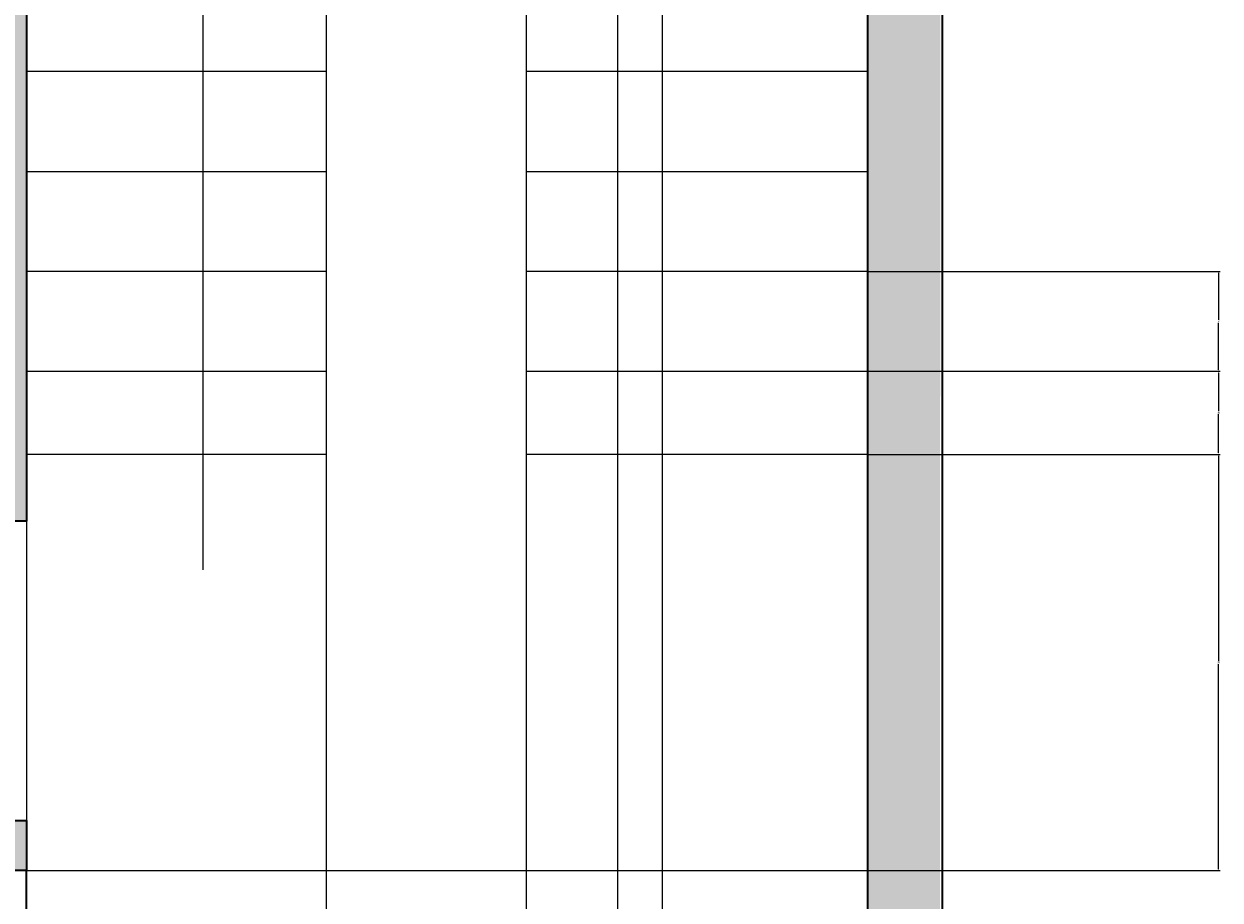
# Model space of a CAD drawing. Units: inches. Extents: x 2070 to 4408, y 1595 to 4269.
# Tile 7 of 20: x 2345 to 2489, y 1739 to 1844. Entities that reach past the tile are written whole.
import ezdxf

# ---------------------------------------------------------------- set-up
doc = ezdxf.new("R2010")
doc.units = ezdxf.units.IN
for name, color, linetype, lineweight in [('A-ANNO-DIMS', 2, 'Continuous', 18), ('A-ANNO-SYMB', 7, 'Continuous', 18), ('A-FLOR-STRS', 7, 'Continuous', 18), ('A-WALL', 7, 'Continuous', 35)]:
    doc.layers.add(name, color=color, linetype=linetype, lineweight=lineweight)
doc.layers.add('A-WALL-PATT', color=18, linetype='Continuous', lineweight=13, true_color=0x000000)
doc.styles.get("Standard").update_dxf_attribs({"font": 'arial.ttf'})
doc.dimstyles.get("Standard").update_dxf_attribs({"dimtxt": 0.18, "dimasz": 0.18, "dimexe": 0.18, "dimexo": 0.0625, "dimgap": 0.09, "dimtad": 0, "dimtih": 1, "dimtoh": 1, "dimdec": 4, "dimzin": 0, "dimdsep": 46, "dimtxsty": 'Standard', "dimcen": 0.09, "dimadec": 0, "dimazin": 0, "dimtfac": 1, "dimtdec": 4, "dimtofl": 0, "dimtmove": 0, "dimatfit": 3, "dimfxl": 1, "dimtolj": 1, "dimtzin": 0, "dimarcsym": 0})

# ---------------------------------------------------------------- blocks, each defined once
blk = doc.blocks.new('*D30')
at = {"layer": 'A-ANNO-DIMS', "color": 0, "lineweight": -2, "transparency": 16777216}
for p, q in [((2416.2, 2080.34), (2416.2, 1595.04)), ((2446.2, 2080.34), (2446.2, 1595.04)), ((2416.38, 1595.22), (2430.98, 1595.22)), ((2446.02, 1595.22), (2431.41, 1595.22))]:
    blk.add_line(p, q, dxfattribs=at)
at = {"layer": 'A-ANNO-DIMS', "color": 0, "transparency": 16777216}
for points in [[(2416.38, 1595.25), (2416.38, 1595.19), (2416.2, 1595.22)], [(2446.02, 1595.25), (2446.02, 1595.19), (2446.2, 1595.22)]]:
    blk.add_solid(points, dxfattribs=at)
at = {"layer": 'Defpoints', "color": 0, "transparency": 16777216}
for p in [(2416.2, 2080.4), (2446.2, 2080.4), (2446.2, 1595.22)]:
    blk.add_point(p, dxfattribs=at)
at = {"layer": 'A-ANNO-DIMS', "color": 0, "transparency": 16777216, "insert": (2431.2, 1595.22), "char_height": 0.18, "attachment_point": 5}
blk.add_mtext('\\A1;30', dxfattribs=at)
blk = doc.blocks.new('*D34')
at = {"layer": 'A-ANNO-DIMS', "color": 0, "lineweight": -2, "transparency": 16777216}
for p, q in [((2421.53, 2212.34), (2421.53, 1595.04)), ((2446.2, 2212.34), (2446.2, 1595.04)), ((2421.71, 1595.22), (2433.4, 1595.22)), ((2446.02, 1595.22), (2434.33, 1595.22))]:
    blk.add_line(p, q, dxfattribs=at)
at = {"layer": 'A-ANNO-DIMS', "color": 0, "transparency": 16777216}
for points in [[(2421.71, 1595.25), (2421.71, 1595.19), (2421.53, 1595.22)], [(2446.02, 1595.25), (2446.02, 1595.19), (2446.2, 1595.22)]]:
    blk.add_solid(points, dxfattribs=at)
at = {"layer": 'Defpoints', "color": 0, "transparency": 16777216}
for p in [(2421.53, 2212.4), (2446.2, 2212.4), (2446.2, 1595.22)]:
    blk.add_point(p, dxfattribs=at)
at = {"layer": 'A-ANNO-DIMS', "color": 0, "transparency": 16777216, "insert": (2433.86, 1595.22), "char_height": 0.18, "attachment_point": 5}
blk.add_mtext('\\A1;24.663', dxfattribs=at)
blk = doc.blocks.new('*D36')
at = {"layer": 'A-ANNO-DIMS', "color": 0, "lineweight": -2, "transparency": 16777216}
for p, q in [((2345.2, 1792.34), (2345.2, 1595.04)), ((2381.2, 1792.34), (2381.2, 1595.04)), ((2345.38, 1595.22), (2362.98, 1595.22)), ((2381.02, 1595.22), (2363.41, 1595.22))]:
    blk.add_line(p, q, dxfattribs=at)
at = {"layer": 'A-ANNO-DIMS', "color": 0, "transparency": 16777216}
for points in [[(2345.38, 1595.25), (2345.38, 1595.19), (2345.2, 1595.22)], [(2381.02, 1595.25), (2381.02, 1595.19), (2381.2, 1595.22)]]:
    blk.add_solid(points, dxfattribs=at)
at = {"layer": 'Defpoints', "color": 0, "transparency": 16777216}
for p in [(2345.2, 1792.4), (2381.2, 1792.4), (2381.2, 1595.22)]:
    blk.add_point(p, dxfattribs=at)
at = {"layer": 'A-ANNO-DIMS', "color": 0, "transparency": 16777216, "insert": (2363.2, 1595.22), "char_height": 0.18, "attachment_point": 5}
blk.add_mtext('\\A1;36', dxfattribs=at)
blk = doc.blocks.new('*D37')
at = {"layer": 'A-ANNO-DIMS', "color": 0, "lineweight": -2, "transparency": 16777216}
for p, q in [((2381.2, 1792.34), (2381.2, 1595.04)), ((2405.2, 1792.34), (2405.2, 1595.04)), ((2381.38, 1595.22), (2392.98, 1595.22)), ((2405.02, 1595.22), (2393.42, 1595.22))]:
    blk.add_line(p, q, dxfattribs=at)
at = {"layer": 'A-ANNO-DIMS', "color": 0, "transparency": 16777216}
for points in [[(2381.38, 1595.25), (2381.38, 1595.19), (2381.2, 1595.22)], [(2405.02, 1595.25), (2405.02, 1595.19), (2405.2, 1595.22)]]:
    blk.add_solid(points, dxfattribs=at)
at = {"layer": 'Defpoints', "color": 0, "transparency": 16777216}
for p in [(2381.2, 1792.4), (2405.2, 1792.4), (2405.2, 1595.22)]:
    blk.add_point(p, dxfattribs=at)
at = {"layer": 'A-ANNO-DIMS', "color": 0, "transparency": 16777216, "insert": (2393.2, 1595.22), "char_height": 0.18, "attachment_point": 5}
blk.add_mtext('\\A1;24', dxfattribs=at)
blk = doc.blocks.new('*D38')
at = {"layer": 'A-ANNO-DIMS', "color": 0, "lineweight": -2, "transparency": 16777216}
for p, q in [((2405.2, 1792.34), (2405.2, 1595.04)), ((2446.2, 1792.34), (2446.2, 1595.04)), ((2405.38, 1595.22), (2425.49, 1595.22)), ((2446.02, 1595.22), (2425.9, 1595.22))]:
    blk.add_line(p, q, dxfattribs=at)
at = {"layer": 'A-ANNO-DIMS', "color": 0, "transparency": 16777216}
for points in [[(2405.38, 1595.25), (2405.38, 1595.19), (2405.2, 1595.22)], [(2446.02, 1595.25), (2446.02, 1595.19), (2446.2, 1595.22)]]:
    blk.add_solid(points, dxfattribs=at)
at = {"layer": 'Defpoints', "color": 0, "transparency": 16777216}
for p in [(2405.2, 1792.4), (2446.2, 1792.4), (2446.2, 1595.22)]:
    blk.add_point(p, dxfattribs=at)
at = {"layer": 'A-ANNO-DIMS', "color": 0, "transparency": 16777216, "insert": (2425.7, 1595.22), "char_height": 0.18, "attachment_point": 5}
blk.add_mtext('\\A1;41', dxfattribs=at)
blk = doc.blocks.new('*D39')
at = {"layer": 'A-ANNO-DIMS', "color": 0, "lineweight": -2, "transparency": 16777216}
for p, q in [((2446.26, 1814.4), (2488.56, 1814.4)), ((2488.38, 1814.22), (2488.38, 1808.58)), ((2488.38, 1802.58), (2488.38, 1808.22)), ((2446.26, 1802.4), (2488.56, 1802.4))]:
    blk.add_line(p, q, dxfattribs=at)
at = {"layer": 'A-ANNO-DIMS', "color": 0, "transparency": 16777216}
for points in [[(2488.35, 1814.22), (2488.41, 1814.22), (2488.38, 1814.4)], [(2488.35, 1802.58), (2488.41, 1802.58), (2488.38, 1802.4)]]:
    blk.add_solid(points, dxfattribs=at)
at = {"layer": 'Defpoints', "color": 0, "transparency": 16777216}
for p in [(2446.2, 1814.4), (2446.2, 1802.4), (2488.38, 1802.4)]:
    blk.add_point(p, dxfattribs=at)
at = {"layer": 'A-ANNO-DIMS', "color": 0, "transparency": 16777216, "insert": (2488.38, 1808.4), "char_height": 0.18, "attachment_point": 5}
blk.add_mtext('\\A1;12', dxfattribs=at)
blk = doc.blocks.new('*D40')
at = {"layer": 'A-ANNO-DIMS', "color": 0, "lineweight": -2, "transparency": 16777216}
for p, q in [((2446.26, 1802.4), (2488.56, 1802.4)), ((2488.38, 1802.22), (2488.38, 1797.58)), ((2488.38, 1792.58), (2488.38, 1797.22)), ((2446.26, 1792.4), (2488.56, 1792.4))]:
    blk.add_line(p, q, dxfattribs=at)
at = {"layer": 'A-ANNO-DIMS', "color": 0, "transparency": 16777216}
for points in [[(2488.35, 1802.22), (2488.41, 1802.22), (2488.38, 1802.4)], [(2488.35, 1792.58), (2488.41, 1792.58), (2488.38, 1792.4)]]:
    blk.add_solid(points, dxfattribs=at)
at = {"layer": 'Defpoints', "color": 0, "transparency": 16777216}
for p in [(2446.2, 1802.4), (2446.2, 1792.4), (2488.38, 1792.4)]:
    blk.add_point(p, dxfattribs=at)
at = {"layer": 'A-ANNO-DIMS', "color": 0, "transparency": 16777216, "insert": (2488.38, 1797.4), "char_height": 0.18, "attachment_point": 5}
blk.add_mtext('\\A1;10', dxfattribs=at)
blk = doc.blocks.new('*D42')
at = {"layer": 'A-ANNO-DIMS', "color": 0, "lineweight": -2, "transparency": 16777216}
for p, q in [((2446.26, 1792.4), (2488.56, 1792.4)), ((2488.38, 1792.22), (2488.38, 1767.58)), ((2488.38, 1742.58), (2488.38, 1767.22)), ((2446.26, 1742.4), (2488.56, 1742.4))]:
    blk.add_line(p, q, dxfattribs=at)
at = {"layer": 'A-ANNO-DIMS', "color": 0, "transparency": 16777216}
for points in [[(2488.35, 1792.22), (2488.41, 1792.22), (2488.38, 1792.4)], [(2488.35, 1742.58), (2488.41, 1742.58), (2488.38, 1742.4)]]:
    blk.add_solid(points, dxfattribs=at)
at = {"layer": 'Defpoints', "color": 0, "transparency": 16777216}
for p in [(2446.2, 1792.4), (2488.38, 1792.4), (2446.2, 1742.4)]:
    blk.add_point(p, dxfattribs=at)
at = {"layer": 'A-ANNO-DIMS', "color": 0, "transparency": 16777216, "insert": (2488.38, 1767.4), "char_height": 0.18, "attachment_point": 5}
blk.add_mtext('\\A1;50', dxfattribs=at)

msp = doc.modelspace()

# ---------------------------------------------------------------- hatches: boundary and pattern name
at = {"layer": 'A-WALL-PATT'}
h = msp.add_hatch(color=256, dxfattribs=at)
h.dxf.hatch_style = 1
h.paths.add_polyline_path([(2346.196, 2218.3995), (2346.196, 2282.3995), (2340.196, 2282.3995), (2340.196, 2212.3995), (2345.5866, 2212.3995), (2346.196, 2212.3995)], flags=0)
h.paths.add_polyline_path([(2245.196, 2282.3995), (2239.196, 2282.3995), (2239.196, 2186.3995), (2244.5866, 2186.3995), (2245.196, 2186.3995)], flags=0)
h.paths.add_polyline_path([(2340.196, 2230.6455), (2245.196, 2230.6455), (2245.196, 2224.6455), (2340.196, 2224.6455)], flags=0)
h.paths.add_polyline_path([(2245.196, 2150.3995), (2239.196, 2150.3995), (2164.4362, 2150.3995), (2164.4362, 2144.3995), (2239.196, 2144.3995), (2239.196, 2086.3995), (2239.196, 2067.2711), (2244.5866, 2067.2711), (2245.196, 2067.2711), (2245.196, 2144.3995)], flags=0)
h.paths.add_polyline_path([(2346.196, 2176.3995), (2340.196, 2176.3995), (2340.196, 2086.3995), (2346.196, 2086.3995), (2346.196, 2125.318)], flags=0)
h.paths.add_polyline_path([(2446.196, 2086.3995), (2346.196, 2086.3995), (2340.196, 2086.3995), (2340.196, 2080.3995), (2446.196, 2080.3995)], flags=0)
h.paths.add_polyline_path([(2455.196, 2291.3995), (2103.196, 2291.3995), (2103.196, 1699.3995), (2336.196, 1699.3995), (2336.196, 1628.3995), (2345.196, 1628.3995), (2446.196, 1628.3995), (2454.8846, 1628.3995), (2454.8846, 1699.3995)])
h.paths.add_polyline_path([(2446.196, 2282.3995), (2446.196, 2218.3995), (2446.196, 2212.3995), (2446.196, 2086.3995), (2446.196, 2080.3995), (2446.196, 1708.3995), (2446.196, 1637.3995), (2345.196, 1637.3995), (2345.196, 1699.3995), (2345.196, 1708.3995), (2336.196, 1708.3995), (2112.196, 1708.3995), (2112.196, 2282.3995), (2239.196, 2282.3995), (2245.196, 2282.3995), (2356.196, 2282.3995)], flags=16)
h.paths.add_polyline_path([(2245.196, 2150.3995), (2245.196, 2144.3995), (2245.196, 2067.2711), (2244.5866, 2067.2711), (2239.196, 2067.2711), (2239.196, 2065.6988), (2203.2929, 2065.6988, 0.40145271), (2239.196, 2031.3337), (2244.5866, 2031.3337), (2245.196, 2031.2711), (2245.196, 1924.1525), (2239.196, 1924.1525), (2239.196, 1922.5803), (2203.2929, 1922.5803, 0.40145271), (2239.196, 1888.2151), (2244.5866, 1888.2151), (2245.196, 1888.1525), (2245.196, 1748.3995), (2339.196, 1748.4621, -0.40145271), (2303.2929, 1782.8272), (2303.2585, 1782.8272), (2303.2585, 1784.3995), (2339.196, 1784.3995), (2339.196, 1877.2067), (2291.196, 1877.2067), (2291.196, 1883.2067), (2291.196, 1946.3995), (2291.196, 1952.3995), (2291.196, 2086.3995), (2297.196, 2086.3995), (2302.196, 2086.3995), (2302.196, 2081.0259), (2303.7633, 2081.0259), (2303.7633, 2080.3995), (2338.0148, 2080.3995, 0.00437129), (2338.0203, 2081.0259), (2338.0203, 2086.3995), (2340.196, 2086.3995), (2340.196, 2176.4621), (2345.5866, 2176.4621, 0.40145271), (2381.4896, 2210.8272), (2345.5866, 2210.8272), (2345.5866, 2212.3995), (2340.196, 2212.3995), (2340.196, 2224.6455), (2245.196, 2224.6455), (2245.196, 2186.3995), (2244.5866, 2186.3995), (2239.196, 2186.3995), (2239.196, 2184.8272), (2203.2929, 2184.8272, 0.40145271), (2239.196, 2150.4621), (2244.5866, 2150.4621)], flags=0)
h.paths.add_polyline_path([(2346.196, 2282.3995), (2346.196, 2218.3995), (2377.1813, 2218.3995), (2377.1813, 2212.3995), (2346.196, 2212.3995), (2345.5866, 2212.3995), (2340.196, 2212.3995), (2340.196, 2224.6455), (2245.196, 2224.6455), (2245.196, 2230.6455), (2245.196, 2282.3995), (2292.696, 2256.5225), (2340.196, 2282.3995)], flags=0)
h.paths.add_polyline_path([(2346.196, 2086.3995), (2340.196, 2086.3995), (2340.196, 2080.3995), (2446.196, 2080.3995), (2431.196, 2016.3995), (2446.196, 1952.3995), (2412.196, 1952.3995), (2412.196, 2080.3995), (2340.196, 2080.3995), (2340.196, 2086.3995), (2340.196, 2176.3995), (2346.196, 2176.3995), (2346.196, 2125.318)], flags=0)
h.paths.add_polyline_path([(2186.508, 2270.0471, -0.03755288), (2186.9712, 2269.8581), (2186.9164, 2270.112, -0.02759121)], flags=0)
h.paths.add_polyline_path([(2183.955, 2273.7766, 1), (2188.2945, 2273.7766, 1)], flags=0)
h.paths.add_polyline_path([(2142.5261, 2274.6158, -0.03707541), (2142.5672, 2275.1696), (2142.5672, 2276.826), (2119.8759, 2276.826), (2119.8759, 2263.0962), (2140.4332, 2263.0962), (2142.5672, 2263.0962), (2142.5672, 2274.0621, -0.03707541)], flags=0)
h.paths.add_polyline_path([(2209.8974, 2263.0962), (2209.8974, 2262.2079), (2190.8042, 2262.2079), (2190.8042, 2263.0962)], flags=0)
h.paths.add_polyline_path([(2210.6382, 2276.1833), (2210.6382, 2263.9844), (2190.2185, 2263.9844), (2190.2185, 2276.1833)], flags=0)
h.paths.add_polyline_path([(2188.4362, 2273.7766, -1), (2183.8133, 2273.7766, -1)], flags=0)
h.paths.add_polyline_path([(2245.196, 2150.3995), (2245.196, 2144.3995), (2245.196, 2067.2711), (2239.196, 2067.2711), (2239.196, 2080.3995), (2172.196, 2080.3995), (2172.196, 2000.3995), (2239.196, 2000.3995), (2239.196, 1940.3995), (2159.0187, 1940.3995), (2123.0187, 1940.3995), (2112.196, 1940.3995), (2112.196, 1946.3995), (2123.0187, 1946.3995), (2123.0187, 1982.2238), (2124.586, 1982.2238), (2124.586, 1982.1895, -0.40145271), (2158.8429, 1946.3995), (2159.0187, 1946.3995), (2239.196, 1946.3995), (2239.196, 1994.3995), (2112.196, 1994.3995), (2112.196, 2000.3995), (2139.196, 2040.3995), (2112.196, 2080.3995), (2112.196, 2086.3995), (2239.196, 2086.3995), (2239.196, 2144.3995), (2209.5809, 2144.3995), (2209.5809, 2136.3995), (2203.0809, 2136.3995), (2205.0809, 2130.3996, -0.70257121), (2199.081, 2116.3995, -0.70256205), (2193.0809, 2130.3994), (2195.0809, 2136.3995), (2192.0809, 2136.3995), (2192.0809, 2134.8995), (2189.0809, 2134.8995), (2189.0809, 2135.8995), (2191.0809, 2135.8995), (2191.0809, 2136.3995), (2188.5809, 2136.3995), (2188.5809, 2144.3995), (2164.2481, 2144.3995, -0.39385849), (2130.0035, 2109.5491), (2130.0035, 2109.5147), (2128.4362, 2109.5147), (2128.4362, 2144.3995), (2112.196, 2144.3995), (2112.196, 2150.3995), (2128.4362, 2150.3995), (2128.4362, 2150.7127), (2164.4362, 2150.7127), (2164.4362, 2150.3995), (2239.196, 2150.3995)], flags=0)
h.paths.add_polyline_path([(2188.2075, 2266.8735), (2188.2075, 2211.8632, -0.41421356), (2185.4833, 2209.1391), (2146.7995, 2209.1391, -0.41421356), (2144.0754, 2211.8632), (2144.0754, 2266.8735, -0.41421356), (2146.7995, 2269.5976), (2185.4833, 2269.5976, -0.41421356)], flags=0)
h.paths.add_polyline_path([(2185.0844, 2273.7766, -1), (2187.1651, 2273.7766, -1)], flags=0)
h.paths.add_polyline_path([(2182.0486, 2259.2932), (2168.0953, 2259.2932), (2168.0953, 2260.8424), (2163.7261, 2260.8424), (2163.7261, 2259.2932), (2149.7727, 2259.2932), (2149.7727, 2266.3352), (2163.7261, 2266.3352), (2163.7261, 2261.9839), (2168.0953, 2261.9839), (2168.0953, 2266.3352), (2182.0486, 2266.3352)], flags=0)
h.paths.add_polyline_path([(2148.2585, 2250.2051), (2153.0615, 2241.8861, 0.39807048)], flags=0)
h.paths.add_polyline_path([(2162.7572, 2247.2885), (2153.1461, 2241.7396), (2148.1083, 2250.4653), (2157.7194, 2256.0142)], flags=0)
h.paths.add_polyline_path([(2162.6726, 2247.4351, -0.39286196), (2157.8415, 2255.6313), (2157.6431, 2255.6313), (2157.8696, 2255.7541)], flags=0)
h.paths.add_polyline_path([(2164.2604, 2145.339), (2164.4362, 2144.3995), (2164.4362, 2150.3995), (2164.2604, 2150.7127)], flags=0)
h.paths.add_polyline_path([(2208.5809, 2142.6495), (2208.5809, 2138.3995, -0.41421356), (2207.8309, 2137.3995), (2190.5809, 2137.3995, -0.41421356), (2189.5809, 2138.1495), (2189.5809, 2142.3995, -0.41421356), (2190.3309, 2143.3995), (2207.5809, 2143.3995, -0.41421356)], flags=0)
h.paths.add_polyline_path([(2147.957, 2229.9119), (2154.7494, 2223.1195, 0.39807048)], flags=0)
h.paths.add_polyline_path([(2162.7165, 2230.8473), (2154.8691, 2222.9998), (2147.7446, 2230.1244), (2155.592, 2237.9718)], flags=0)
h.paths.add_polyline_path([(2162.5969, 2230.9669, -0.39807048), (2155.8044, 2237.7594)], flags=0)
h.paths.add_polyline_path([(2391.8776, 2049.9192), (2408.5766, 2049.9192), (2408.5766, 2033.2202), (2408.5766, 1983.123), (2408.5766, 1966.4239), (2391.8776, 1966.4239), (2391.8776, 1983.123), (2341.7804, 1983.123), (2341.7804, 2033.2202), (2391.8776, 2033.2202)], flags=0)
h.paths.add_polyline_path([(2144.1055, 2274.6158, 1), (2148.445, 2274.6158, 1)], flags=0)
h.paths.add_polyline_path([(2148.5867, 2274.6158, -1), (2143.9638, 2274.6158, -1)], flags=0)
h.paths.add_polyline_path([(2145.2349, 2274.6158, -1), (2147.3156, 2274.6158, -1)], flags=0)
edge = h.paths.add_edge_path(flags=0)
edge.add_ellipse((2400.5951, 2040.9436), major_axis=(-4.5109, 0), ratio=0.97544784, start_angle=180, end_angle=270, ccw=False)
edge.add_ellipse((2400.5951, 2040.9436), major_axis=(-4.5109, 0), ratio=0.97544784, start_angle=90, end_angle=180, ccw=False)
edge.add_ellipse((2400.5951, 2040.9436), major_axis=(-4.5109, 0), ratio=0.97544784, start_angle=0, end_angle=90, ccw=False)
edge.add_ellipse((2400.5951, 2040.9436), major_axis=(-4.5109, 0), ratio=0.97544784, start_angle=270, end_angle=360, ccw=False)
h.paths.add_polyline_path([(2199.0809, 2117.3995, -0.73452973), (2195.0809, 2130.3995), (2203.081, 2130.3995, -0.73453329)], flags=0)
h.paths.add_polyline_path([(2141.9147, 2276.0353), (2141.9147, 2263.9844), (2120.4685, 2263.9844), (2120.4685, 2276.0353)], flags=0)
h.paths.add_polyline_path([(2138.4481, 2273.4072), (2138.4481, 2266.7226), (2133.2801, 2266.7226), (2133.2801, 2273.4072)], flags=0)
h.paths.add_polyline_path([(2137.9691, 2272.9175), (2137.9691, 2272.204), (2135.4229, 2272.204), (2135.4229, 2271.6329), (2135.3221, 2270.1051), (2135.3221, 2269.0265), (2135.4229, 2268.6811), (2135.4229, 2267.2011), (2133.7212, 2267.2011), (2133.7212, 2268.6811), (2133.7983, 2269.9587), (2133.7983, 2271.2758), (2133.7212, 2271.6329), (2133.7212, 2273.0065), (2135.717, 2273.0065), (2135.717, 2272.9175)], flags=0)
h.paths.add_polyline_path([(2137.9215, 2271.8264), (2137.9215, 2271.3786), (2137.5182, 2271.3786), (2136.9355, 2271.3786), (2136.3529, 2271.3786), (2135.7703, 2271.3786), (2135.7703, 2271.8264), (2136.1736, 2271.8264), (2136.7562, 2271.8264), (2137.3389, 2271.8264)], flags=0)
h.paths.add_polyline_path([(2137.9215, 2271.692), (2137.5182, 2271.692), (2136.9355, 2271.513), (2137.3389, 2271.513)], flags=0)
h.paths.add_polyline_path([(2136.3529, 2271.692), (2135.7703, 2271.513), (2136.1736, 2271.513), (2136.7562, 2271.692)], flags=0)
h.paths.add_polyline_path([(2137.9215, 2271.513), (2137.5182, 2271.513), (2136.7562, 2271.747), (2136.7562, 2271.692), (2137.3389, 2271.692)], flags=0)
h.paths.add_polyline_path([(2137.8207, 2270.4664), (2137.8207, 2270.0971), (2137.8207, 2269.627), (2137.8207, 2269.1569), (2137.8207, 2268.6868), (2137.3837, 2268.6868), (2136.6442, 2268.6868), (2135.9271, 2268.6868), (2135.9271, 2269.0562), (2135.9271, 2269.5263), (2135.9271, 2269.9963), (2135.9271, 2270.4664), (2136.3641, 2270.4664), (2137.0812, 2270.4664)], flags=0)
h.paths.add_polyline_path([(2137.3837, 2269.627), (2137.8207, 2269.627), (2137.8207, 2269.5263), (2137.3837, 2269.5263), (2137.3837, 2269.1569), (2137.8207, 2269.1569), (2137.3837, 2269.0562), (2137.3837, 2268.6868), (2137.0812, 2268.6868), (2137.0812, 2269.0562), (2136.6442, 2269.0562), (2136.6442, 2268.6868), (2136.3641, 2268.6868), (2136.3641, 2269.0562), (2135.9271, 2269.0562), (2135.9271, 2269.1569), (2136.3641, 2269.1569), (2136.3641, 2269.5263), (2135.9271, 2269.5263), (2135.9271, 2269.627), (2136.3641, 2269.627), (2136.3641, 2269.9963), (2135.9271, 2269.9963), (2136.3641, 2270.0971), (2136.3641, 2270.4664), (2136.6442, 2270.4664), (2136.6442, 2270.0971), (2137.0812, 2270.0971), (2137.0812, 2270.4664), (2137.3837, 2270.4664), (2137.3837, 2270.0971), (2137.8207, 2270.0971), (2137.3837, 2269.9963)], flags=0)
h.paths.add_polyline_path([(2137.5182, 2271.8264), (2137.5182, 2271.692), (2137.3389, 2271.3786), (2137.3389, 2271.513)], flags=0)
h.paths.add_polyline_path([(2137.8179, 2267.8138), (2137.8179, 2267.6879), (2137.1876, 2267.6879), (2136.4733, 2267.6879), (2135.759, 2267.6879), (2135.759, 2267.8138), (2136.3893, 2267.8138), (2137.1036, 2267.8138)], flags=0)
h.paths.add_polyline_path([(2137.0812, 2269.9963), (2137.0812, 2269.627), (2137.0812, 2269.1569), (2136.6442, 2269.1569), (2136.6442, 2269.5263), (2136.6442, 2269.9963)], flags=0)
h.paths.add_polyline_path([(2136.3529, 2271.8264), (2136.3529, 2271.692), (2136.1736, 2271.3786), (2136.1736, 2271.513)], flags=0)
h.paths.add_polyline_path([(2136.4733, 2267.8138), (2136.4733, 2267.6879), (2136.3893, 2267.6879), (2136.3893, 2267.8138)], flags=0)
h.paths.add_polyline_path([(2407.9087, 2032.5522), (2407.9087, 1983.7909), (2359.81, 1983.7909, -0.00912788), (2359.0575, 1983.7909), (2342.4483, 1983.7909), (2342.4483, 2032.5522)], flags=0)
h.paths.add_polyline_path([(2389.1838, 2023.1358), (2353.7856, 2023.1358), (2353.7856, 1985.4867, -0.09210376), (2350.2788, 1988.655), (2350.2788, 2026.6426), (2389.1838, 2026.6426)], flags=0)
h.paths.add_polyline_path([(2352.6166, 2024.3048), (2351.4477, 2024.3048), (2351.4477, 2025.4737), (2352.6166, 2025.4737)], flags=0)
h.paths.add_polyline_path([(2399.6319, 2026.7589), (2404.3661, 2026.7589, -0.41421356), (2407.0379, 2024.087), (2407.0379, 2013.4908, -0.41421356), (2404.3661, 2010.819), (2399.6319, 2010.819, -0.41421356), (2396.96, 2013.4908), (2396.96, 2024.087, -0.41421356)], flags=0)
h.paths.add_polyline_path([(2399.6319, 2026.0909), (2404.3661, 2026.0909, -0.41421356), (2406.37, 2024.087), (2406.37, 2013.4908, -0.41421356), (2404.3661, 2011.487), (2399.6319, 2011.487, -0.41421356), (2397.628, 2013.4908), (2397.628, 2024.087, -0.41421356)], flags=0)
h.paths.add_polyline_path([(2399.6319, 2002.3217), (2404.3661, 2002.3217, -0.41421356), (2407.0379, 1999.6498), (2407.0379, 1989.0536, -0.41421356), (2404.3661, 1986.3818), (2399.6319, 1986.3818, -0.41421356), (2396.96, 1989.0536), (2396.96, 1999.6498, -0.41421356)], flags=0)
h.paths.add_polyline_path([(2399.6319, 2001.6537), (2404.3661, 2001.6537, -0.41421356), (2406.37, 1999.6498), (2406.37, 1989.0536, -0.41421356), (2404.3661, 1987.0497), (2399.6319, 1987.0497, -0.41421356), (2397.628, 1989.0536), (2397.628, 1999.6498, -0.41421356)], flags=0)
edge = h.paths.add_edge_path(flags=0)
edge.add_ellipse((2400.5951, 1975.3996), major_axis=(-4.5109, 0), ratio=0.97544784, start_angle=-180, end_angle=-90, ccw=False)
edge.add_ellipse((2400.5951, 1975.3996), major_axis=(-4.5109, 0), ratio=0.97544784, start_angle=90, end_angle=180, ccw=False)
edge.add_ellipse((2400.5951, 1975.3996), major_axis=(-4.5109, 0), ratio=0.97544784, start_angle=0, end_angle=90, ccw=False)
edge.add_ellipse((2400.5951, 1975.3996), major_axis=(-4.5109, 0), ratio=0.97544784, start_angle=-90, end_angle=0, ccw=False)
h.paths.add_polyline_path([(2345.196, 1910.3995), (2366.4386, 1910.3995), (2366.4386, 1925.4555), (2392.3856, 1925.4555), (2392.3856, 1933.5025), (2400.1399, 1925.4555), (2392.3856, 1919.8795), (2392.3856, 1925.4555), (2366.4386, 1925.4555), (2366.4386, 1910.3995), (2381.196, 1910.3995), (2405.196, 1910.3995), (2405.196, 1898.3995), (2446.196, 1898.3995), (2446.196, 1886.3995), (2405.196, 1886.3995), (2405.196, 1874.3995), (2446.196, 1874.3995), (2446.196, 1862.3995), (2405.196, 1862.3995), (2405.196, 1850.3995), (2446.196, 1850.3995), (2446.196, 1838.3995), (2405.196, 1838.3995), (2405.196, 1826.3995), (2446.196, 1826.3995), (2446.196, 1814.3995), (2405.196, 1814.3995), (2405.196, 1802.3995), (2446.196, 1802.3995), (2446.196, 1798.3995), (2446.196, 1792.3995), (2405.196, 1792.3995), (2405.196, 1910.3995), (2381.196, 1910.3995), (2381.196, 1792.3995), (2345.196, 1792.3995)], flags=0)
h.paths.add_polyline_path([(2333.0944, 1863.3993, -0.41421356), (2334.7225, 1861.7712), (2334.7225, 1859.329), (2335.2653, 1859.329, -0.41421356), (2337.4361, 1857.1582), (2337.4361, 1843.862, -0.41421356), (2335.2653, 1841.6911, -0.41421356), (2337.4361, 1839.5203), (2337.4361, 1827.5808, -0.41421356), (2335.2653, 1825.41, -0.41421356), (2337.4361, 1823.2392), (2337.4361, 1808.5862, -0.41421356), (2335.2653, 1806.4153), (2334.7225, 1806.4153), (2334.7225, 1803.9732, -0.41421356), (2333.0944, 1802.3451), (2317.356, 1802.3451), (2317.0846, 1802.3451, -0.41421356), (2315.7279, 1803.7018), (2315.7279, 1803.8646), (2313.8284, 1803.8646, -0.41421356), (2311.6576, 1806.0354), (2311.6576, 1823.2015, -0.39597602), (2313.6834, 1825.3765, -0.43384798), (2311.6576, 1827.2718), (2311.6576, 1839.761, -0.41421356), (2313.5571, 1841.6604), (2313.8284, 1841.6604), (2333.8159, 1841.6604, -0.04213623), (2334.1798, 1841.6911, -0.41421356), (2332.009, 1843.862), (2332.009, 1857.1582, -0.41421356), (2334.1798, 1859.329), (2317.356, 1859.329), (2317.0846, 1859.329, -0.41421356), (2315.7279, 1860.6858), (2315.7279, 1862.0426, -0.41421356), (2317.0846, 1863.3993), (2317.356, 1863.3993)], flags=0)
h.paths.add_polyline_path([(2208.8475, 1848.9818), (2208.8475, 1840.9741, -0.41421356), (2207.0458, 1839.1724), (2206.5453, 1839.1721), (2206.5453, 1838.7218, -0.40985861), (2204.7704, 1836.9203), (2183.7501, 1836.9203, -0.41858196), (2181.9216, 1838.7218), (2181.9216, 1839.1721), (2181.421, 1839.1724, -0.41421356), (2179.6193, 1840.9741), (2179.6193, 1848.6817, -0.44064415), (2185.1126, 1854.9874), (2203.3852, 1854.9874, -0.45707961)], flags=0)
h.paths.add_polyline_path([(2204.243, 1848.4815), (2204.243, 1848.4815, 0.41725335), (2202.2204, 1850.4833), (2186.2049, 1850.4833, 0.4111805), (2184.2237, 1848.4815), (2184.2237, 1848.4815, -0.4111807), (2186.2049, 1850.4833), (2202.2204, 1850.4833, -0.41725315)], flags=0)
h.paths.add_polyline_path([(2234.7177, 1830.228), (2234.7176, 1781.6047, -0.41421356), (2233.4381, 1780.3252), (2218.6064, 1780.3252, -0.41421356), (2217.8387, 1781.0929), (2217.8387, 1783.3961, -0.41421356), (2218.6064, 1784.1639), (2218.6065, 1796.9595, -0.41421356), (2219.886, 1798.239, -0.41421356), (2218.6065, 1799.5186), (2218.6065, 1812.3142, -0.41421356), (2219.8861, 1813.5938, -0.41421356), (2218.6065, 1814.8733), (2218.6065, 1827.6689, -0.41421356), (2217.8388, 1828.4367), (2217.8388, 1830.7399, -0.41421356), (2218.6065, 1831.5076), (2233.4382, 1831.5076, -0.41421356)], flags=0)
h.paths.add_polyline_path([(2230.6344, 1827.6689, -0.41421356), (2231.4021, 1826.9012), (2231.4021, 1784.9316, -0.41421356), (2230.6343, 1784.1639), (2221.1853, 1784.1639), (2221.1853, 1827.6689)], flags=0)
h.paths.add_polyline_path([(2222.7208, 1798.239), (2221.6971, 1798.239), (2221.6971, 1813.5938), (2222.7208, 1813.5938)], flags=0)
h.paths.add_polyline_path([(2206.5453, 1773.935), (2206.5453, 1773.4848), (2206.9457, 1773.4848), (2207.0458, 1773.4845, -0.41421356), (2208.8475, 1771.6827), (2208.8475, 1763.675, -0.44222432), (2203.6505, 1757.6695), (2185.3851, 1757.6695, -0.45508402), (2179.6193, 1763.9752), (2179.6193, 1771.6827, -0.41421356), (2181.421, 1773.4845), (2181.421, 1773.4848), (2181.9216, 1773.4848), (2181.9216, 1773.935, -0.40985861), (2183.6965, 1775.7366), (2204.7167, 1775.7366, -0.41858196)], flags=0)
h.paths.add_polyline_path([(2202.2619, 1762.1736), (2186.2464, 1762.1736, -0.41725315), (2184.2237, 1764.1754), (2184.2237, 1764.1754, 0.41725335), (2186.2464, 1762.1736), (2202.2619, 1762.1736, 0.4111805), (2204.243, 1764.1754), (2204.243, 1764.1754, -0.4111807)], flags=0)
h.paths.add_polyline_path([(2313.0034, 1713.1906), (2312.997, 1713.1697), (2313.0123, 1713.1612)], flags=0)
h.paths.add_polyline_path([(2305.7314, 1721.0488), (2305.6257, 1721.1994), (2305.4853, 1721.084)], flags=0)
h.paths.add_polyline_path([(2307.5562, 1726.1427), (2307.6186, 1726.1026), (2307.5737, 1726.0477), (2308.5692, 1720.6434), (2310.5345, 1721.2985), (2310.5721, 1721.411), (2310.6958, 1721.3523), (2313.8453, 1722.4021), (2314.9351, 1723.8033), (2314.9294, 1723.9165), (2315.0028, 1723.8903), (2313.874, 1722.4389), (2313.8697, 1722.4102), (2308.5692, 1720.6434), (2308.9864, 1720.122), (2309.0665, 1720.0971), (2309.053, 1720.0387), (2310.9235, 1717.7005), (2311.4182, 1717.6259), (2311.2918, 1717.2402), (2312.0655, 1716.2731), (2312.1081, 1716.2606), (2312.0969, 1716.2339), (2308.5692, 1720.6434), (2305.2249, 1717.745), (2305.232, 1717.704), (2305.1665, 1717.6944), (2308.5692, 1720.6434)], flags=0)
h.paths.add_polyline_path([(2288.2072, 1714.3431), (2288.2008, 1714.3222), (2288.216, 1714.3137)], flags=0)
h.paths.add_polyline_path([(2280.9352, 1722.2013), (2280.8295, 1722.3519), (2280.689, 1722.2365)], flags=0)
h.paths.add_polyline_path([(2282.76, 1727.2952), (2282.8224, 1727.2551), (2282.7775, 1727.2002), (2283.773, 1721.7959), (2285.7383, 1722.451), (2285.7759, 1722.5635), (2285.8995, 1722.5048), (2289.0491, 1723.5546), (2290.1389, 1724.9558), (2290.1332, 1725.069), (2290.2065, 1725.0428), (2289.0777, 1723.5915), (2289.0735, 1723.5628), (2283.773, 1721.7959), (2284.1901, 1721.2745), (2284.2703, 1721.2496), (2284.2567, 1721.1913), (2286.1273, 1718.8531), (2286.622, 1718.7785), (2286.4956, 1718.3927), (2287.2692, 1717.4256), (2287.3119, 1717.4131), (2287.3006, 1717.3864), (2283.773, 1721.7959), (2280.4286, 1718.8975), (2280.4357, 1718.8565), (2280.3703, 1718.8469), (2283.773, 1721.7959)], flags=0)
h.paths.add_polyline_path([(2302.0672, 1721.8694), (2301.8205, 1721.8572), (2301.7578, 1722.1787), (2299.415, 1724.5215), (2299.103, 1724.4694), (2299.0662, 1724.8703)], flags=0)
h.paths.add_polyline_path([(2264.5643, 1715.4956), (2264.5579, 1715.4747), (2264.5731, 1715.4662)], flags=0)
h.paths.add_polyline_path([(2257.2923, 1723.3538), (2257.1865, 1723.5044), (2257.0461, 1723.389)], flags=0)
h.paths.add_polyline_path([(2259.117, 1728.4477), (2259.1795, 1728.4077), (2259.1345, 1728.3527), (2260.13, 1722.9484), (2262.0954, 1723.6036), (2262.133, 1723.716), (2262.2566, 1723.6573), (2265.4061, 1724.7071), (2266.4959, 1726.1083), (2266.4902, 1726.2215), (2266.5636, 1726.1953), (2265.4348, 1724.744), (2265.4305, 1724.7153), (2260.13, 1722.9484), (2260.5472, 1722.427), (2260.6273, 1722.4022), (2260.6138, 1722.3438), (2262.4843, 1720.0056), (2262.979, 1719.931), (2262.8526, 1719.5452), (2263.6263, 1718.5781), (2263.6689, 1718.5656), (2263.6577, 1718.5389), (2260.13, 1722.9484), (2256.7857, 1720.05), (2256.7928, 1720.009), (2256.7273, 1719.9994), (2260.13, 1722.9484)], flags=0)
h.paths.add_polyline_path([(2277.2709, 1723.0219), (2277.0243, 1723.0097), (2276.9616, 1723.3312), (2274.6187, 1725.6741), (2274.3067, 1725.6219), (2274.27, 1726.0228)], flags=0)
h.paths.add_polyline_path([(2253.628, 1724.1744), (2253.3814, 1724.1622), (2253.3186, 1724.4838), (2250.9758, 1726.8266), (2250.6638, 1726.7744), (2250.627, 1727.1753)], flags=0)
h.paths.add_polyline_path([(2161.9194, 1715.4956), (2161.913, 1715.4747), (2161.9282, 1715.4662)], flags=0)
h.paths.add_polyline_path([(2154.6474, 1723.3538), (2154.5416, 1723.5044), (2154.4012, 1723.389)], flags=0)
h.paths.add_polyline_path([(2162.7899, 1724.744), (2162.7856, 1724.7153), (2157.4851, 1722.9484), (2157.9023, 1722.427), (2157.9824, 1722.4022), (2157.9689, 1722.3438), (2159.8394, 1720.0056), (2160.3341, 1719.931), (2160.2078, 1719.5452), (2160.9814, 1718.5781), (2161.024, 1718.5656), (2161.0128, 1718.5389), (2157.4851, 1722.9484), (2154.1408, 1720.05), (2154.1479, 1720.009), (2154.0824, 1719.9994), (2157.4851, 1722.9484), (2156.4721, 1728.4477), (2156.5346, 1728.4077), (2156.4896, 1728.3527), (2157.4851, 1722.9484), (2159.4505, 1723.6036), (2159.4881, 1723.716), (2159.6117, 1723.6573), (2162.7612, 1724.7071), (2163.851, 1726.1083), (2163.8453, 1726.2215), (2163.9187, 1726.1953)], flags=0)
h.paths.add_polyline_path([(2150.9831, 1724.1744), (2150.7365, 1724.1622), (2150.6738, 1724.4838), (2148.3309, 1726.8266), (2148.0189, 1726.7744), (2147.9822, 1727.1753)], flags=0)
h.paths.add_polyline_path([(2132.5099, 1716.6482), (2132.5035, 1716.6272), (2132.5187, 1716.6187)], flags=0)
h.paths.add_polyline_path([(2125.2379, 1724.5064), (2125.1322, 1724.6569), (2124.9917, 1724.5415)], flags=0)
h.paths.add_polyline_path([(2133.3804, 1725.8965), (2133.3762, 1725.8678), (2128.0757, 1724.101), (2128.4928, 1723.5795), (2128.5729, 1723.5547), (2128.5594, 1723.4963), (2130.43, 1721.1581), (2130.9246, 1721.0835), (2130.7983, 1720.6977), (2131.5719, 1719.7306), (2131.6146, 1719.7181), (2131.6033, 1719.6914), (2128.0757, 1724.101), (2124.7313, 1721.2025), (2124.7384, 1721.1615), (2124.6729, 1721.1519), (2128.0757, 1724.101), (2127.0626, 1729.6002), (2127.1251, 1729.5602), (2127.0801, 1729.5052), (2128.0757, 1724.101), (2130.041, 1724.7561), (2130.0786, 1724.8685), (2130.2022, 1724.8098), (2133.3517, 1725.8597), (2134.4415, 1727.2608), (2134.4358, 1727.3741), (2134.5092, 1727.3478)], flags=0)
h.paths.add_polyline_path([(2121.5736, 1725.3269), (2121.327, 1725.3148), (2121.2643, 1725.6363), (2118.9214, 1727.9791), (2118.6094, 1727.9269), (2118.5727, 1728.3279)], flags=0)
h.paths.add_polyline_path([(2433.3904, 1646.406), (2433.384, 1646.3851), (2433.3992, 1646.3766)], flags=0)
h.paths.add_polyline_path([(2426.1184, 1654.2642), (2426.0127, 1654.4148), (2425.8722, 1654.2994)], flags=0)
h.paths.add_polyline_path([(2427.9432, 1659.3581), (2428.0056, 1659.318), (2427.9606, 1659.2631), (2428.9562, 1653.8588), (2430.9215, 1654.514), (2430.9591, 1654.6264), (2431.0827, 1654.5677), (2434.2323, 1655.6175), (2435.322, 1657.0187), (2435.3163, 1657.1319), (2435.3897, 1657.1057), (2434.2609, 1655.6544), (2434.2567, 1655.6257), (2428.9562, 1653.8588), (2429.3733, 1653.3374), (2429.4534, 1653.3126), (2429.4399, 1653.2542), (2431.3105, 1650.916), (2431.8051, 1650.8414), (2431.6788, 1650.4556), (2432.4524, 1649.4885), (2432.4951, 1649.476), (2432.4838, 1649.4493), (2428.9562, 1653.8588), (2425.6118, 1650.9604), (2425.6189, 1650.9194), (2425.5535, 1650.9098), (2428.9562, 1653.8588)], flags=0)
h.paths.add_polyline_path([(2376.63, 1645.4912), (2376.6236, 1645.4703), (2376.6388, 1645.4617)], flags=0)
h.paths.add_polyline_path([(2369.358, 1653.3494), (2369.2523, 1653.5), (2369.1118, 1653.3845)], flags=0)
h.paths.add_polyline_path([(2371.1828, 1658.4432), (2371.2452, 1658.4032), (2371.2003, 1658.3482), (2372.1958, 1652.944), (2374.1611, 1653.5991), (2374.1987, 1653.7116), (2374.3224, 1653.6528), (2377.4719, 1654.7027), (2378.5617, 1656.1038), (2378.556, 1656.2171), (2378.6293, 1656.1908), (2377.5005, 1654.7395), (2377.4963, 1654.7108), (2372.1958, 1652.944), (2372.6129, 1652.4225), (2372.6931, 1652.3977), (2372.6795, 1652.3393), (2374.5501, 1650.0011), (2375.0448, 1649.9265), (2374.9184, 1649.5407), (2375.692, 1648.5737), (2375.7347, 1648.5611), (2375.7234, 1648.5344), (2372.1958, 1652.944), (2368.8514, 1650.0456), (2368.8586, 1650.0046), (2368.7931, 1649.995), (2372.1958, 1652.944)], flags=0)
h.paths.add_polyline_path([(2404.0947, 1645.0338), (2404.0883, 1645.0128), (2404.1035, 1645.0043)], flags=0)
h.paths.add_polyline_path([(2396.8227, 1652.892), (2396.717, 1653.0425), (2396.5765, 1652.9271)], flags=0)
h.paths.add_polyline_path([(2398.6475, 1657.9858), (2398.7099, 1657.9458), (2398.665, 1657.8908), (2399.6605, 1652.4866), (2401.6258, 1653.1417), (2401.6634, 1653.2541), (2401.7871, 1653.1954), (2404.9366, 1654.2453), (2406.0264, 1655.6464), (2406.0207, 1655.7596), (2406.094, 1655.7334), (2404.9652, 1654.2821), (2404.961, 1654.2534), (2399.6605, 1652.4866), (2400.0776, 1651.9651), (2400.1578, 1651.9403), (2400.1442, 1651.8819), (2402.0148, 1649.5437), (2402.5095, 1649.4691), (2402.3831, 1649.0833), (2403.1567, 1648.1162), (2403.1994, 1648.1037), (2403.1881, 1648.077), (2399.6605, 1652.4866), (2396.3162, 1649.5881), (2396.3233, 1649.5471), (2396.2578, 1649.5375), (2399.6605, 1652.4866)], flags=0)
h.paths.add_polyline_path([(2419.4532, 1658.0857), (2422.4541, 1655.0848), (2422.2075, 1655.0726), (2422.1448, 1655.3941), (2419.8019, 1657.737), (2419.4899, 1657.6848)], flags=0)
h.paths.add_polyline_path([(2390.1575, 1656.7135), (2393.1584, 1653.7125), (2392.9118, 1653.7004), (2392.8491, 1654.0219), (2390.5063, 1656.3647), (2390.1943, 1656.3125)], flags=0)
h.paths.add_polyline_path([(2362.6928, 1657.1709), (2365.6937, 1654.1699), (2365.4471, 1654.1578), (2365.3844, 1654.4793), (2363.0416, 1656.8221), (2362.7295, 1656.77)], flags=0)
h.paths.add_polyline_path([(2419.9523, 2037.8601), (2440.2872, 2037.8601), (2440.2872, 2047.1732), (2419.9523, 2047.1732)], flags=8)
h.paths.add_polyline_path([(2370.186, 1698.9005), (2413.6287, 1698.9005), (2413.6287, 1708.0908), (2370.186, 1708.0908)], flags=8)
h.paths.add_polyline_path([(2370.1656, 1708.5185), (2430.0857, 1708.5185), (2430.0857, 1717.8316), (2370.1656, 1717.8316)], flags=8)
h.paths.add_polyline_path([(2254.1469, 1788.1883), (2302.2471, 1788.1883), (2302.2471, 1797.3786), (2254.1469, 1797.3786)], flags=8)
h.paths.add_polyline_path([(2254.1264, 1797.8063), (2326.1448, 1797.8063), (2326.1448, 1807.1194), (2254.1264, 1807.1194)], flags=8)
h.paths.add_polyline_path([(2300.08, 1914.5069), (2338.861, 1914.5069), (2338.861, 1923.6972), (2300.08, 1923.6972)], flags=8)
h.paths.add_polyline_path([(2300.0595, 1924.1249), (2331.5882, 1924.1249), (2331.5882, 1933.438), (2300.0595, 1933.438)], flags=8)
h.paths.add_polyline_path([(2176.6905, 1716.4567), (2224.1441, 1716.4567), (2224.1441, 1725.647), (2176.6905, 1725.647)], flags=8)
h.paths.add_polyline_path([(2176.67, 1726.0747), (2245.9176, 1726.0747), (2245.9176, 1735.3878), (2176.67, 1735.3878)], flags=8)
h.paths.add_polyline_path([(2339.997, 2039.7696), (2388.1034, 2039.7696), (2388.1034, 2048.9661), (2339.997, 2048.9661)], flags=8)
h.paths.add_polyline_path([(2339.9776, 2049.3928), (2388.7204, 2049.3928), (2388.7204, 2058.7059), (2339.9776, 2058.7059)], flags=8)
h.paths.add_polyline_path([(2366.0063, 2161.3825), (2409.449, 2161.3825), (2409.449, 2170.5728), (2366.0063, 2170.5728)], flags=8)
h.paths.add_polyline_path([(2365.9868, 2171.0016), (2405.879, 2171.0016), (2405.879, 2180.3085), (2365.9868, 2180.3085)], flags=8)
h.paths.add_polyline_path([(2366.0102, 2247.0726), (2407.12, 2247.0726), (2407.12, 2256.263), (2366.0102, 2256.263)], flags=8)
h.paths.add_polyline_path([(2365.9897, 2256.6906), (2397.9686, 2256.6906), (2397.9686, 2266.0037), (2365.9897, 2266.0037)], flags=8)
h.paths.add_polyline_path([(2271.8465, 2102.7885), (2307.6541, 2102.7885), (2307.6541, 2111.9849), (2271.8465, 2111.9849)], flags=8)
h.paths.add_polyline_path([(2271.8281, 2112.4126), (2304.2673, 2112.4126), (2304.2673, 2121.7196), (2271.8281, 2121.7196)], flags=8)
h.paths.add_polyline_path([(2141.6408, 2187.5934), (2182.108, 2187.5934), (2182.108, 2196.7837), (2141.6408, 2196.7837)], flags=8)
h.paths.add_polyline_path([(2141.6203, 2197.2114), (2190.3631, 2197.2114), (2190.3631, 2206.5245), (2141.6203, 2206.5245)], flags=8)
h.paths.add_polyline_path([(2165.7271, 2103.039), (2211.5027, 2103.039), (2211.5027, 2112.2293), (2165.7271, 2112.2293)], flags=8)
h.paths.add_polyline_path([(2165.7077, 2112.658), (2185.1033, 2112.658), (2185.1033, 2121.965), (2165.7077, 2121.965)], flags=8)
h.paths.add_polyline_path([(2174.945, 2048.0789), (2211.3973, 2048.0789), (2211.3973, 2057.2693), (2174.945, 2057.2693)], flags=8)
h.paths.add_polyline_path([(2174.9256, 2057.698), (2194.3212, 2057.698), (2194.3212, 2067.0049), (2174.9256, 2067.0049)], flags=8)
h.paths.add_polyline_path([(2164.8305, 1965.8394), (2202.9649, 1965.8394), (2202.9649, 1975.0297), (2164.8305, 1975.0297)], flags=8)
h.paths.add_polyline_path([(2164.8111, 1975.4584), (2184.2067, 1975.4584), (2184.2067, 1984.7654), (2164.8111, 1984.7654)], flags=8)
h.paths.add_polyline_path([(2133.0392, 1862.086), (2173.5065, 1862.086), (2173.5065, 1871.2763), (2133.0392, 1871.2763)], flags=8)
h.paths.add_polyline_path([(2133.0709, 1871.8585), (2157.0382, 1871.8585), (2157.0382, 1880.8585), (2133.0709, 1880.8585)], flags=8)
h.paths.add_polyline_path([(2406.4423, 1923.5541), (2418.8209, 1923.5541), (2418.8209, 1932.7199), (2406.4423, 1932.7199)], flags=8)
h = msp.add_hatch(color=256, dxfattribs=at)
h.dxf.hatch_style = 1
h.paths.add_polyline_path([(2245.196, 2282.3995), (2239.196, 2282.3995), (2239.196, 2186.3995), (2244.5866, 2186.3995), (2245.196, 2186.3995)])
h.paths.add_polyline_path([(2340.196, 2230.6455), (2245.196, 2230.6455), (2245.196, 2224.6455), (2340.196, 2224.6455)])
h.paths.add_polyline_path([(2346.196, 2282.3995), (2340.196, 2282.3995), (2340.196, 2212.3995), (2345.5866, 2212.3995), (2346.196, 2212.3995), (2346.196, 2218.3995)])
h.paths.add_polyline_path([(2245.196, 2144.3995), (2245.196, 2150.3995), (2239.196, 2150.3995), (2164.4362, 2150.3995), (2164.4362, 2144.3995), (2239.196, 2144.3995), (2239.196, 2086.3995), (2239.196, 2067.2711), (2244.5866, 2067.2711), (2245.196, 2067.2711)])
h.paths.add_polyline_path([(2128.4362, 2150.3995), (2112.196, 2150.3995), (2112.196, 2144.3995), (2128.4362, 2144.3995), (2128.4362, 2145.339)])
h.paths.add_polyline_path([(2239.196, 2086.3995), (2112.196, 2086.3995), (2112.196, 2080.3995), (2239.196, 2080.3995)])
h.paths.add_polyline_path([(2172.196, 2080.3995), (2166.196, 2080.3995), (2166.196, 2000.3995), (2172.196, 2000.3995)])
h.paths.add_polyline_path([(2239.196, 2000.3995), (2112.196, 2000.3995), (2112.196, 1994.3995), (2239.196, 1994.3995)])
h.paths.add_polyline_path([(2245.196, 2031.2711), (2239.196, 2031.2711), (2239.196, 2000.3995), (2239.196, 1940.3995), (2245.196, 1940.3995)])
h.paths.add_polyline_path([(2239.196, 1946.3995), (2159.0187, 1946.3995), (2159.0187, 1940.3995), (2239.196, 1940.3995)])
h.paths.add_polyline_path([(2123.0187, 1946.3995), (2112.196, 1946.3995), (2112.196, 1940.3995), (2123.0187, 1940.3995)])
h.paths.add_polyline_path([(2377.1813, 2218.3995), (2346.196, 2218.3995), (2346.196, 2212.3995), (2377.1813, 2212.3995)])
h.paths.add_polyline_path([(2446.196, 2218.3995), (2413.1813, 2218.3995), (2413.1813, 2212.3995), (2446.196, 2212.3995)])
h.paths.add_polyline_path([(2446.196, 2086.3995), (2346.196, 2086.3995), (2340.196, 2086.3995), (2340.196, 2080.3995), (2446.196, 2080.3995)], flags=17)
h.paths.add_polyline_path([(2346.196, 2125.318), (2346.196, 2176.3995), (2340.196, 2176.3995), (2340.196, 2086.3995), (2346.196, 2086.3995)])
h.paths.add_polyline_path([(2245.196, 1888.1525), (2239.196, 1888.1525), (2239.196, 1748.3995), (2245.196, 1748.3995)])
h.paths.add_polyline_path([(2345.196, 1748.3995), (2239.196, 1748.3995), (2112.196, 1748.3995), (2112.196, 1742.3995), (2239.196, 1742.3995), (2345.196, 1742.3995)])
h.paths.add_polyline_path([(2297.196, 2080.3995), (2297.196, 2086.3995), (2291.196, 2086.3995), (2291.196, 1952.3995), (2291.196, 1946.3995), (2339.196, 1946.3995), (2339.196, 1883.2067), (2291.196, 1883.2067), (2291.196, 1877.2067), (2339.196, 1877.2067), (2339.196, 1784.3995), (2345.196, 1784.3995), (2345.196, 1792.3995), (2345.196, 1946.3995), (2446.196, 1946.3995), (2446.196, 1952.3995), (2297.196, 1952.3995)])

# ---------------------------------------------------------------- linework, layer by layer
at = {"layer": 'A-ANNO-SYMB'}
msp.add_line((2366.4386, 1778.524), (2366.4386, 1925.4555), dxfattribs=at)
at = {"layer": 'A-FLOR-STRS'}
for p, q in [((2381.196, 1910.3995), (2381.196, 1792.3995)), ((2405.196, 1910.3995), (2405.196, 1792.3995)), ((2446.196, 1850.3995), (2446.196, 1838.3995)), ((2345.196, 1838.3995), (2345.196, 1826.3995)), ((2381.196, 1838.3995), (2345.196, 1838.3995)), ((2446.196, 1838.3995), (2405.196, 1838.3995)), ((2345.196, 1826.3995), (2381.196, 1826.3995)), ((2405.196, 1826.3995), (2446.196, 1826.3995)), ((2446.196, 1826.3995), (2446.196, 1814.3995)), ((2345.196, 1814.3995), (2345.196, 1802.3995)), ((2381.196, 1814.3995), (2345.196, 1814.3995)), ((2446.196, 1814.3995), (2405.196, 1814.3995)), ((2345.196, 1802.3995), (2381.196, 1802.3995)), ((2405.196, 1802.3995), (2446.196, 1802.3995)), ((2446.196, 1802.3995), (2446.196, 1798.3995)), ((2446.196, 1798.3995), (2446.196, 1792.3995)), ((2345.196, 1792.3995), (2345.196, 1784.3995)), ((2381.196, 1792.3995), (2345.196, 1792.3995)), ((2446.196, 1792.3995), (2405.196, 1792.3995)), ((2446.196, 1784.3995), (2446.196, 1776.3995)), ((2345.196, 1742.3995), (2446.196, 1742.3995))]:
    msp.add_line(p, q, dxfattribs=at)
at = {"layer": 'A-WALL'}
for p, q in [((2345.196, 1946.3995), (2345.196, 1784.3995)), ((2345.196, 1784.3995), (2339.196, 1784.3995)), ((2239.196, 1748.3995), (2345.196, 1748.3995)), ((2345.196, 1748.3995), (2345.196, 1742.3995)), ((2345.196, 1748.3995), (2345.196, 1742.3995)), ((2345.196, 1742.3995), (2239.196, 1742.3995)), ((2345.196, 1742.3995), (2336.196, 1742.3995)), ((2345.196, 1708.3995), (2345.196, 1742.3995))]:
    msp.add_line(p, q, dxfattribs=at)
for points in [[(2336.196, 1699.3995), (2103.196, 1699.3995), (2103.196, 2291.3995), (2455.196, 2291.3995), (2455.196, 1699.3995), (2454.8846, 1699.3995)], [(2446.196, 2212.3995), (2446.196, 1708.3995)]]:
    msp.add_lwpolyline(points, dxfattribs=at)

# ---------------------------------------------------------------- dimensions: what is measured, and where the dimension line sits
at = {"layer": 'A-ANNO-DIMS'}
for base, p1, p2, override, picture, middle in [((2446.196, 1595.2195), (2421.5333, 2212.3995), (2446.196, 2212.3995), {"dimdec": 3, "dimlfac": 1, "dimrnd": 0, "dimzin": 0, "dimdsep": 46, "dimlunit": 2}, '*D34', (2433.8646, 1595.2195)), ((2446.196, 1595.2195), (2416.196, 2080.3995), (2446.196, 2080.3995), {"dimdec": 0, "dimlfac": 1, "dimrnd": 0, "dimzin": 0, "dimdsep": 46, "dimlunit": 2}, '*D30', (2431.196, 1595.2195)), ((2381.196, 1595.2195), (2345.196, 1792.3995), (2381.196, 1792.3995), {"dimdec": 0, "dimlfac": 1, "dimrnd": 0, "dimzin": 0, "dimdsep": 46, "dimlunit": 2}, '*D36', (2363.196, 1595.2195)), ((2405.196, 1595.2195), (2381.196, 1792.3995), (2405.196, 1792.3995), {"dimdec": 0, "dimlfac": 1, "dimrnd": 0, "dimzin": 0, "dimdsep": 46, "dimlunit": 2}, '*D37', (2393.196, 1595.2195)), ((2446.196, 1595.2195), (2405.196, 1792.3995), (2446.196, 1792.3995), {"dimdec": 0, "dimlfac": 1, "dimrnd": 0, "dimzin": 0, "dimdsep": 46, "dimlunit": 2}, '*D38', (2425.696, 1595.2195))]:
    dim = msp.add_linear_dim(base=base, p1=p1, p2=p2, dimstyle='Standard', override=override, dxfattribs=at)
    dim.commit()
    dim.dimension.update_dxf_attribs({"geometry": picture, "text_midpoint": middle})
for base, p1, p2, picture, middle in [((2488.376, 1802.3995), (2446.196, 1814.3995), (2446.196, 1802.3995), '*D39', (2488.376, 1808.3995)), ((2488.376, 1792.3995), (2446.196, 1802.3995), (2446.196, 1792.3995), '*D40', (2488.376, 1797.3995)), ((2488.376, 1792.3995), (2446.196, 1742.3995), (2446.196, 1792.3995), '*D42', (2488.376, 1767.3995))]:
    dim = msp.add_linear_dim(base=base, p1=p1, p2=p2, angle=90, dimstyle='Standard', override={"dimdec": 0, "dimlfac": 1, "dimrnd": 0, "dimzin": 0, "dimdsep": 46, "dimlunit": 2}, dxfattribs=at)
    dim.commit()
    dim.dimension.update_dxf_attribs({"geometry": picture, "text_midpoint": middle})

doc.saveas('drawing.dxf')
